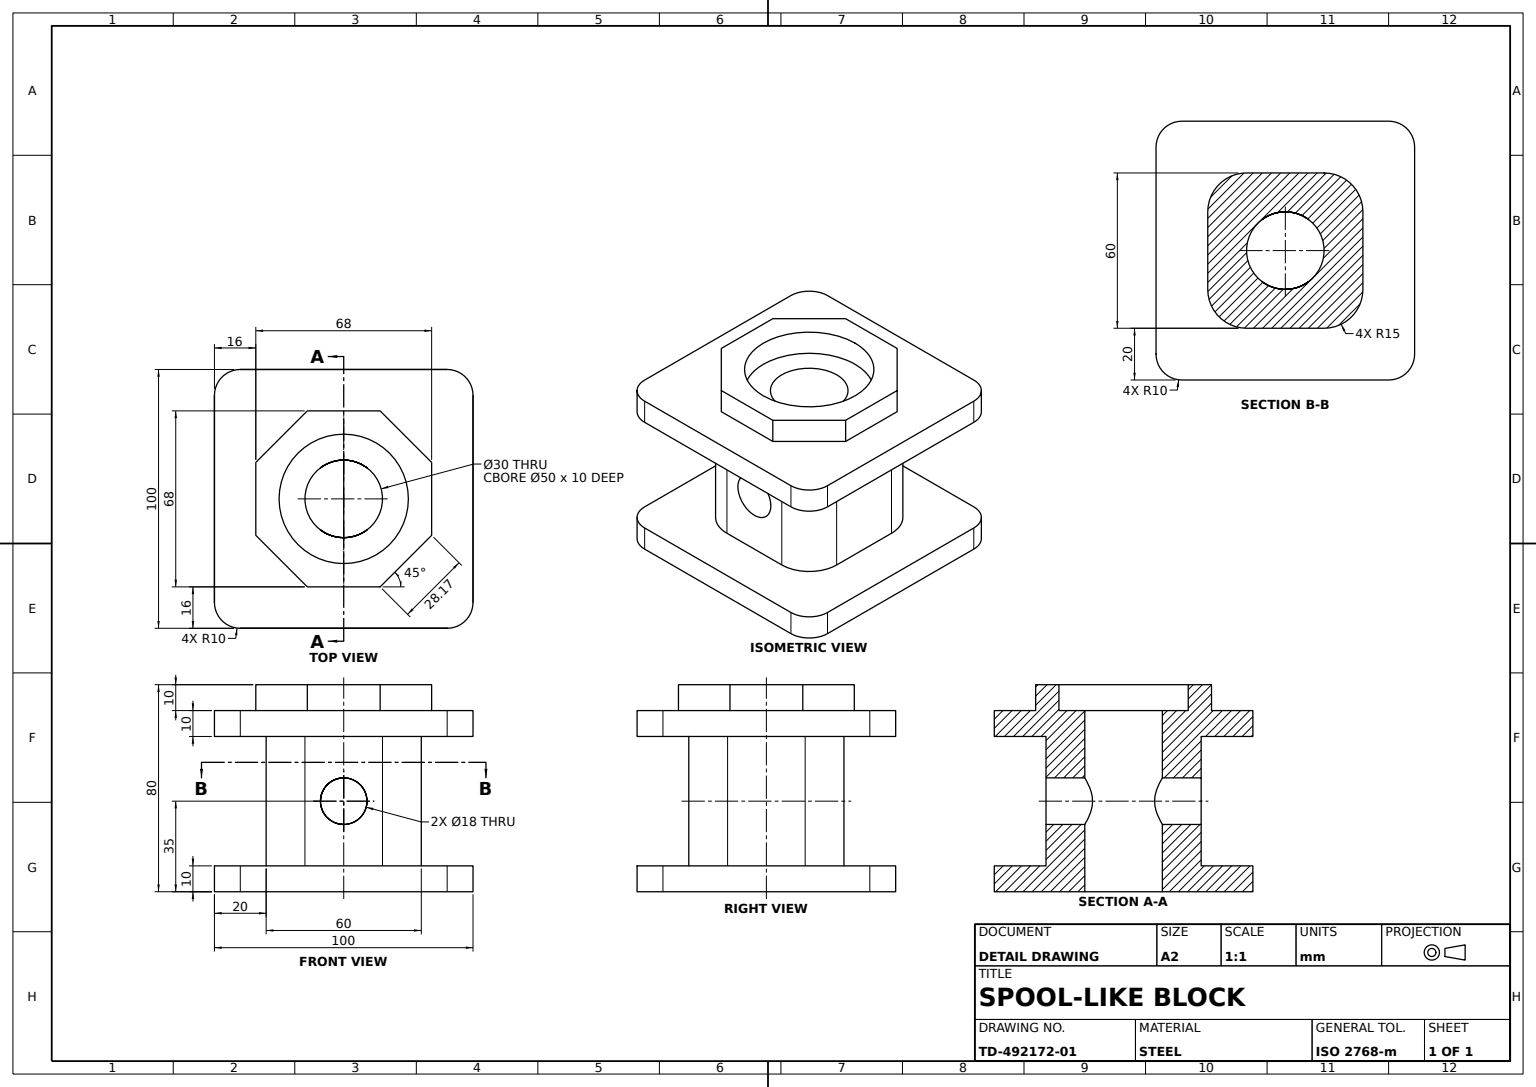
from build123d import *

# Parameters (mm, degrees)
BASE_PLATE_SKETCH_R    = 15
BASE_PLATE_DEPTH       = 10
CENTRE_COLUMN_SKETCH_R = 15
CENTRE_COLUMN_DEPTH    = 50
TOP_PLATE_SKETCH_R     = 15
TOP_PLATE_DEPTH        = 10
OCTAGON_BOSS_SKETCH_R  = 25
OCTAGON_BOSS_DEPTH     = 10
CROSS_HOLE_18_D        = 18


with BuildPart() as part:
    # Base Plate Sketch → Base Plate (new body)
    with BuildSketch(Plane(origin=(0, 0, 0), x_dir=(1, 0, 0), z_dir=(0, 1, 0))):
        with BuildLine():
            Line((-40, 50), (40, 50))
            ThreePointArc((40, 50), (47.071067812, 47.071067812), (50, 40))
            Line((50, 40), (50, -40))
            ThreePointArc((50, -40), (47.071067812, -47.071067812), (40, -50))
            Line((40, -50), (-40, -50))
            ThreePointArc((-40, -50), (-47.071067812, -47.071067812), (-50, -40))
            Line((-50, -40), (-50, 40))
            ThreePointArc((-50, 40), (-47.071067812, 47.071067812), (-40, 50))
        make_face()
        with Locations(Location((0, 0, 0), (0, 0, 270))):
            Circle(BASE_PLATE_SKETCH_R, mode=Mode.SUBTRACT)
    extrude(amount=BASE_PLATE_DEPTH)

    # Centre Column Sketch → Centre Column (add)
    with BuildSketch(Plane(origin=(0, 10, 0), x_dir=(1, 0, 0), z_dir=(0, 1, 0))):
        with BuildLine():
            Line((-15, 30), (15, 30))
            ThreePointArc((15, 30), (25.606601718, 25.606601718), (30, 15))
            Line((30, 15), (30, -15))
            ThreePointArc((30, -15), (25.606601718, -25.606601718), (15, -30))
            Line((15, -30), (-15, -30))
            ThreePointArc((-15, -30), (-25.606601718, -25.606601718), (-30, -15))
            Line((-30, -15), (-30, 15))
            ThreePointArc((-30, 15), (-25.606601718, 25.606601718), (-15, 30))
        make_face()
        with Locations(Location((0, 0, 0), (0, 0, 270))):
            Circle(CENTRE_COLUMN_SKETCH_R, mode=Mode.SUBTRACT)
    extrude(amount=CENTRE_COLUMN_DEPTH)

    # Top Plate Sketch → Top Plate (add)
    with BuildSketch(Plane(origin=(0, 60, 0), x_dir=(1, 0, 0), z_dir=(0, 1, 0))):
        with BuildLine():
            Line((-40, -50), (40, -50))
            ThreePointArc((40, -50), (47.071067812, -47.071067812), (50, -40))
            Line((50, -40), (50, 40))
            ThreePointArc((50, 40), (47.071067812, 47.071067812), (40, 50))
            Line((40, 50), (-40, 50))
            ThreePointArc((-40, 50), (-47.071067812, 47.071067812), (-50, 40))
            Line((-50, 40), (-50, -40))
            ThreePointArc((-50, -40), (-47.071067812, -47.071067812), (-40, -50))
        make_face()
        with Locations(Location((0, 0, 0), (0, 0, 270))):
            Circle(TOP_PLATE_SKETCH_R, mode=Mode.SUBTRACT)
    extrude(amount=TOP_PLATE_DEPTH)

    # Octagon Boss Sketch → Octagon Boss (add)
    with BuildSketch(Plane(origin=(0, 70, 0), x_dir=(1, 0, 0), z_dir=(0, 1, 0))):
        Polygon((34, -14.083261121), (34, 14.083261121), (14.083261121, 34), (-14.083261121, 34), (-34, 14.083261121), (-34, -14.083261121), (-14.083261121, -34), (14.083261121, -34), align=None)
        with Locations(Location((0, 0, 0), (0, 0, 270))):
            Circle(OCTAGON_BOSS_SKETCH_R, mode=Mode.SUBTRACT)
    extrude(amount=OCTAGON_BOSS_DEPTH)

    # Cross Hole Ø18 (through all)
    with Locations(Plane.XY.offset(30)):
        with Locations((0, 35)):
            Hole(CROSS_HOLE_18_D / 2)


solid = part.part
